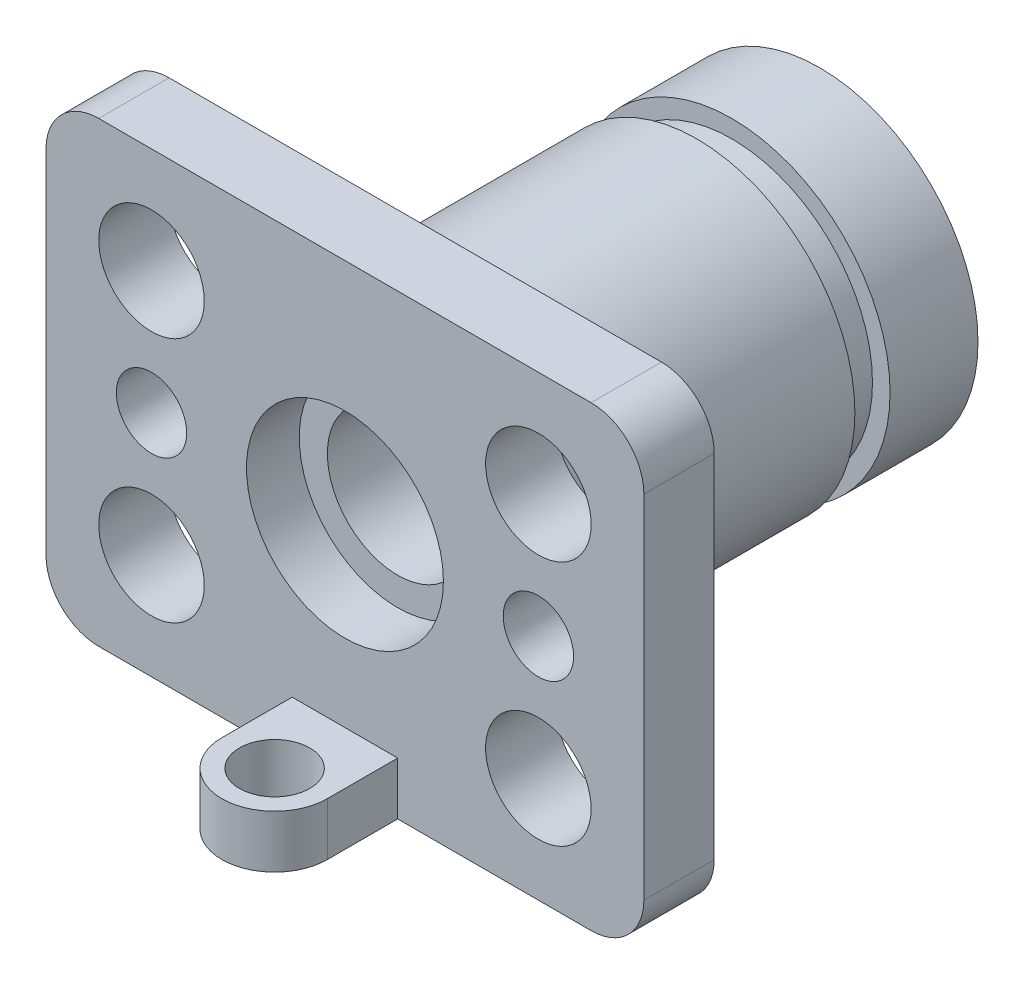
ISO-10303-21;
HEADER;
FILE_DESCRIPTION(('STEP AP214'),'2;1');
FILE_NAME('part.step','',(''),(''),'','','');
FILE_SCHEMA(('AUTOMOTIVE_DESIGN { 1 0 10303 214 1 1 1 1 }'));
ENDSEC;
DATA;
#1=APPLICATION_CONTEXT('core data for automotive mechanical design processes');
#2=APPLICATION_PROTOCOL_DEFINITION('international standard','automotive_design',2000,#1);
#3=PRODUCT_CONTEXT('',#1,'mechanical');
#4=PRODUCT('Part','Part','',(#3));
#5=PRODUCT_RELATED_PRODUCT_CATEGORY('part','',(#4));
#6=PRODUCT_DEFINITION_FORMATION('','',#4);
#7=PRODUCT_DEFINITION_CONTEXT('part definition',#1,'design');
#8=PRODUCT_DEFINITION('design','',#6,#7);
#9=PRODUCT_DEFINITION_SHAPE('','',#8);
#10=(LENGTH_UNIT() NAMED_UNIT(*) SI_UNIT(.MILLI.,.METRE.));
#11=(NAMED_UNIT(*) PLANE_ANGLE_UNIT() SI_UNIT($,.RADIAN.));
#12=(NAMED_UNIT(*) SI_UNIT($,.STERADIAN.) SOLID_ANGLE_UNIT());
#13=UNCERTAINTY_MEASURE_WITH_UNIT(LENGTH_MEASURE(1.E-05),#10,'distance_accuracy_value','');
#14=(GEOMETRIC_REPRESENTATION_CONTEXT(3) GLOBAL_UNCERTAINTY_ASSIGNED_CONTEXT((#13)) GLOBAL_UNIT_ASSIGNED_CONTEXT((#10,
#11,#12)) REPRESENTATION_CONTEXT('',''));
#15=CARTESIAN_POINT('',(0.,0.,0.));
#16=DIRECTION('',(0.,0.,1.));
#17=DIRECTION('',(1.,0.,0.));
#18=AXIS2_PLACEMENT_3D('',#15,#16,#17);
#19=CARTESIAN_POINT('',(0.,0.,25.));
#20=DIRECTION('',(0.,0.,-1.));
#21=DIRECTION('',(-1.,0.,0.));
#22=AXIS2_PLACEMENT_3D('',#19,#20,#21);
#23=CYLINDRICAL_SURFACE('',#22,45.);
#24=CARTESIAN_POINT('',(0.,0.,25.));
#25=DIRECTION('',(0.,0.,1.));
#26=DIRECTION('',(1.,0.,0.));
#27=AXIS2_PLACEMENT_3D('',#24,#25,#26);
#28=CIRCLE('',#27,45.);
#29=CARTESIAN_POINT('',(45.,0.,25.));
#30=VERTEX_POINT('',#29);
#31=EDGE_CURVE('E54',#30,#30,#28,.T.);
#32=ORIENTED_EDGE('',*,*,#31,.F.);
#33=EDGE_LOOP('',(#32));
#34=FACE_BOUND('',#33,.T.);
#35=CARTESIAN_POINT('',(0.,0.,0.));
#36=DIRECTION('',(0.,0.,1.));
#37=DIRECTION('',(1.,0.,0.));
#38=AXIS2_PLACEMENT_3D('',#35,#36,#37);
#39=CIRCLE('',#38,45.);
#40=CARTESIAN_POINT('',(45.,0.,0.));
#41=VERTEX_POINT('',#40);
#42=EDGE_CURVE('E284',#41,#41,#39,.T.);
#43=ORIENTED_EDGE('',*,*,#42,.T.);
#44=EDGE_LOOP('',(#43));
#45=FACE_BOUND('',#44,.T.);
#46=ADVANCED_FACE('F50',(#34,#45),#23,.T.);
#47=CARTESIAN_POINT('',(0.,0.,25.));
#48=DIRECTION('',(0.,0.,1.));
#49=DIRECTION('',(1.,0.,0.));
#50=AXIS2_PLACEMENT_3D('',#47,#48,#49);
#51=PLANE('',#50);
#52=CARTESIAN_POINT('',(0.,0.,25.));
#53=DIRECTION('',(0.,0.,1.));
#54=DIRECTION('',(1.,0.,0.));
#55=AXIS2_PLACEMENT_3D('',#52,#53,#54);
#56=CIRCLE('',#55,40.);
#57=CARTESIAN_POINT('',(40.,0.,25.));
#58=VERTEX_POINT('',#57);
#59=EDGE_CURVE('E11',#58,#58,#56,.T.);
#60=ORIENTED_EDGE('',*,*,#59,.F.);
#61=EDGE_LOOP('',(#60));
#62=FACE_BOUND('',#61,.T.);
#63=ORIENTED_EDGE('',*,*,#31,.T.);
#64=EDGE_LOOP('',(#63));
#65=FACE_BOUND('',#64,.T.);
#66=ADVANCED_FACE('F326',(#62,#65),#51,.T.);
#67=CARTESIAN_POINT('',(0.,0.,0.));
#68=DIRECTION('',(0.,0.,1.));
#69=DIRECTION('',(1.,0.,0.));
#70=AXIS2_PLACEMENT_3D('',#67,#68,#69);
#71=PLANE('',#70);
#72=CARTESIAN_POINT('',(0.,0.,0.));
#73=DIRECTION('',(0.,0.,1.));
#74=DIRECTION('',(1.,0.,0.));
#75=AXIS2_PLACEMENT_3D('',#72,#73,#74);
#76=CIRCLE('',#75,20.);
#77=CARTESIAN_POINT('',(20.,0.,0.));
#78=VERTEX_POINT('',#77);
#79=EDGE_CURVE('E202',#78,#78,#76,.T.);
#80=ORIENTED_EDGE('',*,*,#79,.T.);
#81=EDGE_LOOP('',(#80));
#82=FACE_BOUND('',#81,.T.);
#83=ORIENTED_EDGE('',*,*,#42,.F.);
#84=EDGE_LOOP('',(#83));
#85=FACE_BOUND('',#84,.T.);
#86=ADVANCED_FACE('F335',(#82,#85),#71,.F.);
#87=CARTESIAN_POINT('',(0.,0.,35.));
#88=DIRECTION('',(0.,0.,-1.));
#89=DIRECTION('',(-1.,0.,0.));
#90=AXIS2_PLACEMENT_3D('',#87,#88,#89);
#91=CYLINDRICAL_SURFACE('',#90,40.);
#92=CARTESIAN_POINT('',(0.,0.,35.));
#93=DIRECTION('',(0.,0.,1.));
#94=DIRECTION('',(1.,0.,0.));
#95=AXIS2_PLACEMENT_3D('',#92,#93,#94);
#96=CIRCLE('',#95,40.);
#97=CARTESIAN_POINT('',(40.,0.,35.));
#98=VERTEX_POINT('',#97);
#99=EDGE_CURVE('E279',#98,#98,#96,.T.);
#100=ORIENTED_EDGE('',*,*,#99,.F.);
#101=EDGE_LOOP('',(#100));
#102=FACE_BOUND('',#101,.T.);
#103=ORIENTED_EDGE('',*,*,#59,.T.);
#104=EDGE_LOOP('',(#103));
#105=FACE_BOUND('',#104,.T.);
#106=ADVANCED_FACE('F340',(#102,#105),#91,.T.);
#107=CARTESIAN_POINT('',(0.,0.,115.));
#108=DIRECTION('',(0.,0.,-1.));
#109=DIRECTION('',(-1.,0.,0.));
#110=AXIS2_PLACEMENT_3D('',#107,#108,#109);
#111=CYLINDRICAL_SURFACE('',#110,45.);
#112=CARTESIAN_POINT('',(0.,0.,115.));
#113=DIRECTION('',(0.,0.,1.));
#114=DIRECTION('',(1.,0.,0.));
#115=AXIS2_PLACEMENT_3D('',#112,#113,#114);
#116=CIRCLE('',#115,45.);
#117=CARTESIAN_POINT('',(45.,0.,115.));
#118=VERTEX_POINT('',#117);
#119=CARTESIAN_POINT('',(-45.,0.,115.));
#120=VERTEX_POINT('',#119);
#121=EDGE_CURVE('E274',#118,#120,#116,.T.);
#122=ORIENTED_EDGE('',*,*,#121,.F.);
#123=EDGE_CURVE('E276',#120,#118,#116,.T.);
#124=ORIENTED_EDGE('',*,*,#123,.F.);
#125=EDGE_LOOP('',(#122,#124));
#126=FACE_BOUND('',#125,.T.);
#127=CARTESIAN_POINT('',(0.,0.,35.));
#128=DIRECTION('',(0.,0.,1.));
#129=DIRECTION('',(1.,0.,0.));
#130=AXIS2_PLACEMENT_3D('',#127,#128,#129);
#131=CIRCLE('',#130,45.);
#132=CARTESIAN_POINT('',(45.,0.,35.));
#133=VERTEX_POINT('',#132);
#134=EDGE_CURVE('E273',#133,#133,#131,.T.);
#135=ORIENTED_EDGE('',*,*,#134,.T.);
#136=EDGE_LOOP('',(#135));
#137=FACE_BOUND('',#136,.T.);
#138=ADVANCED_FACE('F347',(#126,#137),#111,.T.);
#139=CARTESIAN_POINT('',(0.,0.,35.));
#140=DIRECTION('',(0.,0.,1.));
#141=DIRECTION('',(1.,0.,0.));
#142=AXIS2_PLACEMENT_3D('',#139,#140,#141);
#143=PLANE('',#142);
#144=ORIENTED_EDGE('',*,*,#99,.T.);
#145=EDGE_LOOP('',(#144));
#146=FACE_BOUND('',#145,.T.);
#147=ORIENTED_EDGE('',*,*,#134,.F.);
#148=EDGE_LOOP('',(#147));
#149=FACE_BOUND('',#148,.T.);
#150=ADVANCED_FACE('F351',(#146,#149),#143,.F.);
#151=CARTESIAN_POINT('',(70.,50.,135.));
#152=DIRECTION('',(0.,0.,-1.));
#153=DIRECTION('',(-1.,0.,0.));
#154=AXIS2_PLACEMENT_3D('',#151,#152,#153);
#155=CYLINDRICAL_SURFACE('',#154,15.);
#156=CARTESIAN_POINT('',(70.,50.,115.));
#157=DIRECTION('',(0.,0.,1.));
#158=DIRECTION('',(1.,0.,0.));
#159=AXIS2_PLACEMENT_3D('',#156,#157,#158);
#160=CIRCLE('',#159,15.);
#161=CARTESIAN_POINT('',(85.,49.9999999999999,115.));
#162=VERTEX_POINT('',#161);
#163=CARTESIAN_POINT('',(69.9999999999999,65.,115.));
#164=VERTEX_POINT('',#163);
#165=EDGE_CURVE('E207',#162,#164,#160,.T.);
#166=ORIENTED_EDGE('',*,*,#165,.T.);
#167=DIRECTION('',(0.,0.,-1.));
#168=VECTOR('',#167,1.);
#169=CARTESIAN_POINT('',(69.9999999999999,65.,135.));
#170=LINE('',#169,#168);
#171=CARTESIAN_POINT('',(69.9999999999999,65.,135.));
#172=VERTEX_POINT('',#171);
#173=EDGE_CURVE('E275',#172,#164,#170,.T.);
#174=ORIENTED_EDGE('',*,*,#173,.F.);
#175=CARTESIAN_POINT('',(70.,50.,135.));
#176=DIRECTION('',(0.,0.,1.));
#177=DIRECTION('',(1.,0.,0.));
#178=AXIS2_PLACEMENT_3D('',#175,#176,#177);
#179=CIRCLE('',#178,15.);
#180=CARTESIAN_POINT('',(85.,49.9999999999999,135.));
#181=VERTEX_POINT('',#180);
#182=EDGE_CURVE('E213',#181,#172,#179,.T.);
#183=ORIENTED_EDGE('',*,*,#182,.F.);
#184=DIRECTION('',(0.,0.,-1.));
#185=VECTOR('',#184,1.);
#186=CARTESIAN_POINT('',(85.,49.9999999999999,135.));
#187=LINE('',#186,#185);
#188=EDGE_CURVE('E237',#181,#162,#187,.T.);
#189=ORIENTED_EDGE('',*,*,#188,.T.);
#190=EDGE_LOOP('',(#166,#174,#183,#189));
#191=FACE_BOUND('',#190,.T.);
#192=ADVANCED_FACE('F355',(#191),#155,.T.);
#193=CARTESIAN_POINT('',(0.,65.,135.));
#194=DIRECTION('',(0.,1.,0.));
#195=DIRECTION('',(0.,0.,1.));
#196=AXIS2_PLACEMENT_3D('',#193,#194,#195);
#197=PLANE('',#196);
#198=DIRECTION('',(1.,0.,0.));
#199=VECTOR('',#198,1.);
#200=CARTESIAN_POINT('',(0.,65.,115.));
#201=LINE('',#200,#199);
#202=CARTESIAN_POINT('',(-69.9999999999999,65.,115.));
#203=VERTEX_POINT('',#202);
#204=EDGE_CURVE('E239',#203,#164,#201,.T.);
#205=ORIENTED_EDGE('',*,*,#204,.F.);
#206=DIRECTION('',(0.,0.,-1.));
#207=VECTOR('',#206,1.);
#208=CARTESIAN_POINT('',(-69.9999999999999,65.,135.));
#209=LINE('',#208,#207);
#210=CARTESIAN_POINT('',(-69.9999999999999,65.,135.));
#211=VERTEX_POINT('',#210);
#212=EDGE_CURVE('E269',#211,#203,#209,.T.);
#213=ORIENTED_EDGE('',*,*,#212,.F.);
#214=DIRECTION('',(1.,0.,0.));
#215=VECTOR('',#214,1.);
#216=CARTESIAN_POINT('',(0.,65.,135.));
#217=LINE('',#216,#215);
#218=EDGE_CURVE('E214',#211,#172,#217,.T.);
#219=ORIENTED_EDGE('',*,*,#218,.T.);
#220=ORIENTED_EDGE('',*,*,#173,.T.);
#221=EDGE_LOOP('',(#205,#213,#219,#220));
#222=FACE_BOUND('',#221,.T.);
#223=ADVANCED_FACE('F359',(#222),#197,.T.);
#224=CARTESIAN_POINT('',(-70.,50.,135.));
#225=DIRECTION('',(0.,0.,-1.));
#226=DIRECTION('',(-1.,0.,0.));
#227=AXIS2_PLACEMENT_3D('',#224,#225,#226);
#228=CYLINDRICAL_SURFACE('',#227,15.);
#229=CARTESIAN_POINT('',(-70.,50.,115.));
#230=DIRECTION('',(0.,0.,1.));
#231=DIRECTION('',(1.,0.,0.));
#232=AXIS2_PLACEMENT_3D('',#229,#230,#231);
#233=CIRCLE('',#232,15.);
#234=CARTESIAN_POINT('',(-85.,49.9999999999999,115.));
#235=VERTEX_POINT('',#234);
#236=EDGE_CURVE('E242',#203,#235,#233,.T.);
#237=ORIENTED_EDGE('',*,*,#236,.T.);
#238=DIRECTION('',(0.,0.,-1.));
#239=VECTOR('',#238,1.);
#240=CARTESIAN_POINT('',(-85.,49.9999999999999,135.));
#241=LINE('',#240,#239);
#242=CARTESIAN_POINT('',(-85.,49.9999999999999,135.));
#243=VERTEX_POINT('',#242);
#244=EDGE_CURVE('E268',#243,#235,#241,.T.);
#245=ORIENTED_EDGE('',*,*,#244,.F.);
#246=CARTESIAN_POINT('',(-70.,50.,135.));
#247=DIRECTION('',(0.,0.,1.));
#248=DIRECTION('',(1.,0.,0.));
#249=AXIS2_PLACEMENT_3D('',#246,#247,#248);
#250=CIRCLE('',#249,15.);
#251=EDGE_CURVE('E218',#211,#243,#250,.T.);
#252=ORIENTED_EDGE('',*,*,#251,.F.);
#253=ORIENTED_EDGE('',*,*,#212,.T.);
#254=EDGE_LOOP('',(#237,#245,#252,#253));
#255=FACE_BOUND('',#254,.T.);
#256=ADVANCED_FACE('F361',(#255),#228,.T.);
#257=CARTESIAN_POINT('',(-85.,0.,135.));
#258=DIRECTION('',(-1.,0.,0.));
#259=DIRECTION('',(0.,0.,1.));
#260=AXIS2_PLACEMENT_3D('',#257,#258,#259);
#261=PLANE('',#260);
#262=DIRECTION('',(0.,1.,0.));
#263=VECTOR('',#262,1.);
#264=CARTESIAN_POINT('',(-85.,0.,115.));
#265=LINE('',#264,#263);
#266=CARTESIAN_POINT('',(-85.,-49.9999999999999,115.));
#267=VERTEX_POINT('',#266);
#268=EDGE_CURVE('E245',#267,#235,#265,.T.);
#269=ORIENTED_EDGE('',*,*,#268,.F.);
#270=DIRECTION('',(0.,0.,-1.));
#271=VECTOR('',#270,1.);
#272=CARTESIAN_POINT('',(-85.,-49.9999999999999,135.));
#273=LINE('',#272,#271);
#274=CARTESIAN_POINT('',(-85.,-49.9999999999999,135.));
#275=VERTEX_POINT('',#274);
#276=EDGE_CURVE('E266',#275,#267,#273,.T.);
#277=ORIENTED_EDGE('',*,*,#276,.F.);
#278=DIRECTION('',(0.,1.,0.));
#279=VECTOR('',#278,1.);
#280=CARTESIAN_POINT('',(-85.,0.,135.));
#281=LINE('',#280,#279);
#282=EDGE_CURVE('E222',#275,#243,#281,.T.);
#283=ORIENTED_EDGE('',*,*,#282,.T.);
#284=ORIENTED_EDGE('',*,*,#244,.T.);
#285=EDGE_LOOP('',(#269,#277,#283,#284));
#286=FACE_BOUND('',#285,.T.);
#287=ADVANCED_FACE('F370',(#286),#261,.T.);
#288=CARTESIAN_POINT('',(-70.,-50.,135.));
#289=DIRECTION('',(0.,0.,-1.));
#290=DIRECTION('',(-1.,0.,0.));
#291=AXIS2_PLACEMENT_3D('',#288,#289,#290);
#292=CYLINDRICAL_SURFACE('',#291,15.);
#293=CARTESIAN_POINT('',(-70.,-50.,115.));
#294=DIRECTION('',(0.,0.,1.));
#295=DIRECTION('',(1.,0.,0.));
#296=AXIS2_PLACEMENT_3D('',#293,#294,#295);
#297=CIRCLE('',#296,15.);
#298=CARTESIAN_POINT('',(-69.9999999999999,-65.,115.));
#299=VERTEX_POINT('',#298);
#300=EDGE_CURVE('E246',#299,#267,#297,.F.);
#301=ORIENTED_EDGE('',*,*,#300,.F.);
#302=DIRECTION('',(0.,0.,-1.));
#303=VECTOR('',#302,1.);
#304=CARTESIAN_POINT('',(-69.9999999999999,-65.,135.));
#305=LINE('',#304,#303);
#306=CARTESIAN_POINT('',(-69.9999999999999,-65.,135.));
#307=VERTEX_POINT('',#306);
#308=EDGE_CURVE('E262',#307,#299,#305,.T.);
#309=ORIENTED_EDGE('',*,*,#308,.F.);
#310=CARTESIAN_POINT('',(-70.,-50.,135.));
#311=DIRECTION('',(0.,0.,1.));
#312=DIRECTION('',(1.,0.,0.));
#313=AXIS2_PLACEMENT_3D('',#310,#311,#312);
#314=CIRCLE('',#313,15.);
#315=EDGE_CURVE('E221',#307,#275,#314,.F.);
#316=ORIENTED_EDGE('',*,*,#315,.T.);
#317=ORIENTED_EDGE('',*,*,#276,.T.);
#318=EDGE_LOOP('',(#301,#309,#316,#317));
#319=FACE_BOUND('',#318,.T.);
#320=ADVANCED_FACE('F371',(#319),#292,.T.);
#321=CARTESIAN_POINT('',(0.,-65.,135.));
#322=DIRECTION('',(0.,-1.,0.));
#323=DIRECTION('',(0.,0.,-1.));
#324=AXIS2_PLACEMENT_3D('',#321,#322,#323);
#325=PLANE('',#324);
#326=CARTESIAN_POINT('',(0.,-65.,155.));
#327=DIRECTION('',(0.,1.,0.));
#328=DIRECTION('',(0.,0.,1.));
#329=AXIS2_PLACEMENT_3D('',#326,#327,#328);
#330=CIRCLE('',#329,10.);
#331=CARTESIAN_POINT('',(0.,-65.,165.));
#332=VERTEX_POINT('',#331);
#333=EDGE_CURVE('E180',#332,#332,#330,.T.);
#334=ORIENTED_EDGE('',*,*,#333,.T.);
#335=EDGE_LOOP('',(#334));
#336=FACE_BOUND('',#335,.T.);
#337=DIRECTION('',(-1.,0.,0.));
#338=VECTOR('',#337,1.);
#339=CARTESIAN_POINT('',(0.,-65.,115.));
#340=LINE('',#339,#338);
#341=CARTESIAN_POINT('',(69.9999999999999,-65.,115.));
#342=VERTEX_POINT('',#341);
#343=EDGE_CURVE('E253',#342,#299,#340,.T.);
#344=ORIENTED_EDGE('',*,*,#343,.F.);
#345=DIRECTION('',(0.,0.,-1.));
#346=VECTOR('',#345,1.);
#347=CARTESIAN_POINT('',(69.9999999999999,-65.,135.));
#348=LINE('',#347,#346);
#349=CARTESIAN_POINT('',(69.9999999999999,-65.,135.));
#350=VERTEX_POINT('',#349);
#351=EDGE_CURVE('E265',#350,#342,#348,.T.);
#352=ORIENTED_EDGE('',*,*,#351,.F.);
#353=DIRECTION('',(-1.,0.,0.));
#354=VECTOR('',#353,1.);
#355=CARTESIAN_POINT('',(0.,-65.,135.));
#356=LINE('',#355,#354);
#357=CARTESIAN_POINT('',(15.,-65.,135.));
#358=VERTEX_POINT('',#357);
#359=EDGE_CURVE('E229',#350,#358,#356,.T.);
#360=ORIENTED_EDGE('',*,*,#359,.T.);
#361=DIRECTION('',(0.,0.,1.));
#362=VECTOR('',#361,1.);
#363=CARTESIAN_POINT('',(15.,-65.,155.));
#364=LINE('',#363,#362);
#365=CARTESIAN_POINT('',(15.,-65.,155.));
#366=VERTEX_POINT('',#365);
#367=EDGE_CURVE('E64',#358,#366,#364,.T.);
#368=ORIENTED_EDGE('',*,*,#367,.T.);
#369=CARTESIAN_POINT('',(0.,-65.,155.));
#370=DIRECTION('',(0.,-1.,0.));
#371=DIRECTION('',(0.,0.,-1.));
#372=AXIS2_PLACEMENT_3D('',#369,#370,#371);
#373=CIRCLE('',#372,15.);
#374=CARTESIAN_POINT('',(-15.,-65.,155.));
#375=VERTEX_POINT('',#374);
#376=EDGE_CURVE('E175',#366,#375,#373,.T.);
#377=ORIENTED_EDGE('',*,*,#376,.T.);
#378=DIRECTION('',(0.,0.,-1.));
#379=VECTOR('',#378,1.);
#380=CARTESIAN_POINT('',(-15.,-65.,155.));
#381=LINE('',#380,#379);
#382=CARTESIAN_POINT('',(-15.,-65.,135.));
#383=VERTEX_POINT('',#382);
#384=EDGE_CURVE('E146',#375,#383,#381,.T.);
#385=ORIENTED_EDGE('',*,*,#384,.T.);
#386=EDGE_CURVE('E227',#383,#307,#356,.T.);
#387=ORIENTED_EDGE('',*,*,#386,.T.);
#388=ORIENTED_EDGE('',*,*,#308,.T.);
#389=EDGE_LOOP('',(#344,#352,#360,#368,#377,#385,#387,#388));
#390=FACE_BOUND('',#389,.T.);
#391=ADVANCED_FACE('F374',(#336,#390),#325,.T.);
#392=CARTESIAN_POINT('',(70.,-50.,135.));
#393=DIRECTION('',(0.,0.,-1.));
#394=DIRECTION('',(-1.,0.,0.));
#395=AXIS2_PLACEMENT_3D('',#392,#393,#394);
#396=CYLINDRICAL_SURFACE('',#395,15.);
#397=CARTESIAN_POINT('',(70.,-50.,115.));
#398=DIRECTION('',(0.,0.,1.));
#399=DIRECTION('',(1.,0.,0.));
#400=AXIS2_PLACEMENT_3D('',#397,#398,#399);
#401=CIRCLE('',#400,15.);
#402=CARTESIAN_POINT('',(85.,-49.9999999999999,115.));
#403=VERTEX_POINT('',#402);
#404=EDGE_CURVE('E255',#342,#403,#401,.T.);
#405=ORIENTED_EDGE('',*,*,#404,.T.);
#406=DIRECTION('',(0.,0.,-1.));
#407=VECTOR('',#406,1.);
#408=CARTESIAN_POINT('',(85.,-49.9999999999999,135.));
#409=LINE('',#408,#407);
#410=CARTESIAN_POINT('',(85.,-49.9999999999999,135.));
#411=VERTEX_POINT('',#410);
#412=EDGE_CURVE('E257',#411,#403,#409,.T.);
#413=ORIENTED_EDGE('',*,*,#412,.F.);
#414=CARTESIAN_POINT('',(70.,-50.,135.));
#415=DIRECTION('',(0.,0.,1.));
#416=DIRECTION('',(1.,0.,0.));
#417=AXIS2_PLACEMENT_3D('',#414,#415,#416);
#418=CIRCLE('',#417,15.);
#419=EDGE_CURVE('E233',#350,#411,#418,.T.);
#420=ORIENTED_EDGE('',*,*,#419,.F.);
#421=ORIENTED_EDGE('',*,*,#351,.T.);
#422=EDGE_LOOP('',(#405,#413,#420,#421));
#423=FACE_BOUND('',#422,.T.);
#424=ADVANCED_FACE('F377',(#423),#396,.T.);
#425=CARTESIAN_POINT('',(85.,0.,135.));
#426=DIRECTION('',(1.,0.,0.));
#427=DIRECTION('',(0.,0.,-1.));
#428=AXIS2_PLACEMENT_3D('',#425,#426,#427);
#429=PLANE('',#428);
#430=DIRECTION('',(0.,-1.,0.));
#431=VECTOR('',#430,1.);
#432=CARTESIAN_POINT('',(85.,0.,115.));
#433=LINE('',#432,#431);
#434=EDGE_CURVE('E216',#162,#403,#433,.T.);
#435=ORIENTED_EDGE('',*,*,#434,.F.);
#436=ORIENTED_EDGE('',*,*,#188,.F.);
#437=DIRECTION('',(0.,-1.,0.));
#438=VECTOR('',#437,1.);
#439=CARTESIAN_POINT('',(85.,0.,135.));
#440=LINE('',#439,#438);
#441=EDGE_CURVE('E231',#181,#411,#440,.T.);
#442=ORIENTED_EDGE('',*,*,#441,.T.);
#443=ORIENTED_EDGE('',*,*,#412,.T.);
#444=EDGE_LOOP('',(#435,#436,#442,#443));
#445=FACE_BOUND('',#444,.T.);
#446=ADVANCED_FACE('F382',(#445),#429,.T.);
#447=CARTESIAN_POINT('',(0.,0.,135.));
#448=DIRECTION('',(0.,0.,1.));
#449=DIRECTION('',(1.,0.,0.));
#450=AXIS2_PLACEMENT_3D('',#447,#448,#449);
#451=PLANE('',#450);
#452=DIRECTION('',(0.,-1.,0.));
#453=VECTOR('',#452,1.);
#454=CARTESIAN_POINT('',(-15.,-50.,135.));
#455=LINE('',#454,#453);
#456=CARTESIAN_POINT('',(-15.,-50.,135.));
#457=VERTEX_POINT('',#456);
#458=EDGE_CURVE('E153',#457,#383,#455,.T.);
#459=ORIENTED_EDGE('',*,*,#458,.F.);
#460=DIRECTION('',(1.,0.,0.));
#461=VECTOR('',#460,1.);
#462=CARTESIAN_POINT('',(-15.,-50.,135.));
#463=LINE('',#462,#461);
#464=CARTESIAN_POINT('',(15.,-50.,135.));
#465=VERTEX_POINT('',#464);
#466=EDGE_CURVE('E162',#457,#465,#463,.T.);
#467=ORIENTED_EDGE('',*,*,#466,.T.);
#468=DIRECTION('',(0.,-1.,0.));
#469=VECTOR('',#468,1.);
#470=CARTESIAN_POINT('',(15.,-50.,135.));
#471=LINE('',#470,#469);
#472=EDGE_CURVE('E182',#465,#358,#471,.T.);
#473=ORIENTED_EDGE('',*,*,#472,.T.);
#474=ORIENTED_EDGE('',*,*,#359,.F.);
#475=ORIENTED_EDGE('',*,*,#419,.T.);
#476=ORIENTED_EDGE('',*,*,#441,.F.);
#477=ORIENTED_EDGE('',*,*,#182,.T.);
#478=ORIENTED_EDGE('',*,*,#218,.F.);
#479=ORIENTED_EDGE('',*,*,#251,.T.);
#480=ORIENTED_EDGE('',*,*,#282,.F.);
#481=ORIENTED_EDGE('',*,*,#315,.F.);
#482=ORIENTED_EDGE('',*,*,#386,.F.);
#483=EDGE_LOOP('',(#459,#467,#473,#474,#475,#476,#477,#478,#479,#480,#481,#482));
#484=FACE_BOUND('',#483,.T.);
#485=CARTESIAN_POINT('',(55.,35.,135.));
#486=DIRECTION('',(0.,0.,1.));
#487=DIRECTION('',(1.,0.,0.));
#488=AXIS2_PLACEMENT_3D('',#485,#486,#487);
#489=CIRCLE('',#488,15.);
#490=CARTESIAN_POINT('',(70.,35.,135.));
#491=VERTEX_POINT('',#490);
#492=EDGE_CURVE('E177',#491,#491,#489,.T.);
#493=ORIENTED_EDGE('',*,*,#492,.F.);
#494=EDGE_LOOP('',(#493));
#495=FACE_BOUND('',#494,.T.);
#496=CARTESIAN_POINT('',(55.,0.,135.));
#497=DIRECTION('',(0.,0.,1.));
#498=DIRECTION('',(1.,0.,0.));
#499=AXIS2_PLACEMENT_3D('',#496,#497,#498);
#500=CIRCLE('',#499,10.);
#501=CARTESIAN_POINT('',(65.,0.,135.));
#502=VERTEX_POINT('',#501);
#503=EDGE_CURVE('E194',#502,#502,#500,.T.);
#504=ORIENTED_EDGE('',*,*,#503,.F.);
#505=EDGE_LOOP('',(#504));
#506=FACE_BOUND('',#505,.T.);
#507=CARTESIAN_POINT('',(55.,-35.,135.));
#508=DIRECTION('',(0.,0.,1.));
#509=DIRECTION('',(1.,0.,0.));
#510=AXIS2_PLACEMENT_3D('',#507,#508,#509);
#511=CIRCLE('',#510,15.);
#512=CARTESIAN_POINT('',(70.,-35.,135.));
#513=VERTEX_POINT('',#512);
#514=EDGE_CURVE('E193',#513,#513,#511,.T.);
#515=ORIENTED_EDGE('',*,*,#514,.F.);
#516=EDGE_LOOP('',(#515));
#517=FACE_BOUND('',#516,.T.);
#518=CARTESIAN_POINT('',(-55.,-35.,135.));
#519=DIRECTION('',(0.,0.,1.));
#520=DIRECTION('',(1.,0.,0.));
#521=AXIS2_PLACEMENT_3D('',#518,#519,#520);
#522=CIRCLE('',#521,15.);
#523=CARTESIAN_POINT('',(-40.,-35.,135.));
#524=VERTEX_POINT('',#523);
#525=EDGE_CURVE('E189',#524,#524,#522,.T.);
#526=ORIENTED_EDGE('',*,*,#525,.F.);
#527=EDGE_LOOP('',(#526));
#528=FACE_BOUND('',#527,.T.);
#529=CARTESIAN_POINT('',(-55.,0.,135.));
#530=DIRECTION('',(0.,0.,1.));
#531=DIRECTION('',(1.,0.,0.));
#532=AXIS2_PLACEMENT_3D('',#529,#530,#531);
#533=CIRCLE('',#532,10.);
#534=CARTESIAN_POINT('',(-45.,0.,135.));
#535=VERTEX_POINT('',#534);
#536=EDGE_CURVE('E184',#535,#535,#533,.T.);
#537=ORIENTED_EDGE('',*,*,#536,.F.);
#538=EDGE_LOOP('',(#537));
#539=FACE_BOUND('',#538,.T.);
#540=CARTESIAN_POINT('',(-55.,35.,135.));
#541=DIRECTION('',(0.,0.,1.));
#542=DIRECTION('',(1.,0.,0.));
#543=AXIS2_PLACEMENT_3D('',#540,#541,#542);
#544=CIRCLE('',#543,15.);
#545=CARTESIAN_POINT('',(-40.,35.,135.));
#546=VERTEX_POINT('',#545);
#547=EDGE_CURVE('E187',#546,#546,#544,.T.);
#548=ORIENTED_EDGE('',*,*,#547,.F.);
#549=EDGE_LOOP('',(#548));
#550=FACE_BOUND('',#549,.T.);
#551=CARTESIAN_POINT('',(0.,0.,135.));
#552=DIRECTION('',(0.,0.,1.));
#553=DIRECTION('',(1.,0.,0.));
#554=AXIS2_PLACEMENT_3D('',#551,#552,#553);
#555=CIRCLE('',#554,28.);
#556=CARTESIAN_POINT('',(28.,0.,135.));
#557=VERTEX_POINT('',#556);
#558=EDGE_CURVE('E209',#557,#557,#555,.T.);
#559=ORIENTED_EDGE('',*,*,#558,.F.);
#560=EDGE_LOOP('',(#559));
#561=FACE_BOUND('',#560,.T.);
#562=ADVANCED_FACE('F390',(#484,#495,#506,#517,#528,#539,#550,#561),#451,.T.);
#563=CARTESIAN_POINT('',(0.,0.,115.));
#564=DIRECTION('',(0.,0.,1.));
#565=DIRECTION('',(1.,0.,0.));
#566=AXIS2_PLACEMENT_3D('',#563,#564,#565);
#567=PLANE('',#566);
#568=CARTESIAN_POINT('',(55.,35.,115.));
#569=DIRECTION('',(0.,0.,1.));
#570=DIRECTION('',(1.,0.,0.));
#571=AXIS2_PLACEMENT_3D('',#568,#569,#570);
#572=CIRCLE('',#571,15.);
#573=CARTESIAN_POINT('',(70.,35.,115.));
#574=VERTEX_POINT('',#573);
#575=EDGE_CURVE('E49',#574,#574,#572,.T.);
#576=ORIENTED_EDGE('',*,*,#575,.T.);
#577=EDGE_LOOP('',(#576));
#578=FACE_BOUND('',#577,.T.);
#579=CARTESIAN_POINT('',(55.,-35.,115.));
#580=DIRECTION('',(0.,0.,1.));
#581=DIRECTION('',(1.,0.,0.));
#582=AXIS2_PLACEMENT_3D('',#579,#580,#581);
#583=CIRCLE('',#582,15.);
#584=CARTESIAN_POINT('',(70.,-35.,115.));
#585=VERTEX_POINT('',#584);
#586=EDGE_CURVE('E297',#585,#585,#583,.T.);
#587=ORIENTED_EDGE('',*,*,#586,.T.);
#588=EDGE_LOOP('',(#587));
#589=FACE_BOUND('',#588,.T.);
#590=CARTESIAN_POINT('',(-55.,-35.,115.));
#591=DIRECTION('',(0.,0.,1.));
#592=DIRECTION('',(1.,0.,0.));
#593=AXIS2_PLACEMENT_3D('',#590,#591,#592);
#594=CIRCLE('',#593,15.);
#595=CARTESIAN_POINT('',(-40.,-35.,115.));
#596=VERTEX_POINT('',#595);
#597=EDGE_CURVE('E294',#596,#596,#594,.T.);
#598=ORIENTED_EDGE('',*,*,#597,.T.);
#599=EDGE_LOOP('',(#598));
#600=FACE_BOUND('',#599,.T.);
#601=CARTESIAN_POINT('',(-55.,35.,115.));
#602=DIRECTION('',(0.,0.,1.));
#603=DIRECTION('',(1.,0.,0.));
#604=AXIS2_PLACEMENT_3D('',#601,#602,#603);
#605=CIRCLE('',#604,15.);
#606=CARTESIAN_POINT('',(-40.,35.,115.));
#607=VERTEX_POINT('',#606);
#608=EDGE_CURVE('E203',#607,#607,#605,.T.);
#609=ORIENTED_EDGE('',*,*,#608,.T.);
#610=EDGE_LOOP('',(#609));
#611=FACE_BOUND('',#610,.T.);
#612=ORIENTED_EDGE('',*,*,#123,.T.);
#613=CARTESIAN_POINT('',(55.,0.,115.));
#614=DIRECTION('',(0.,0.,1.));
#615=DIRECTION('',(1.,0.,0.));
#616=AXIS2_PLACEMENT_3D('',#613,#614,#615);
#617=CIRCLE('',#616,10.);
#618=EDGE_CURVE('E298',#118,#118,#617,.T.);
#619=ORIENTED_EDGE('',*,*,#618,.T.);
#620=ORIENTED_EDGE('',*,*,#121,.T.);
#621=CARTESIAN_POINT('',(-55.,0.,115.));
#622=DIRECTION('',(0.,0.,1.));
#623=DIRECTION('',(1.,0.,0.));
#624=AXIS2_PLACEMENT_3D('',#621,#622,#623);
#625=CIRCLE('',#624,10.);
#626=EDGE_CURVE('E69',#120,#120,#625,.T.);
#627=ORIENTED_EDGE('',*,*,#626,.T.);
#628=EDGE_LOOP('',(#612,#619,#620,#627));
#629=FACE_BOUND('',#628,.T.);
#630=ORIENTED_EDGE('',*,*,#165,.F.);
#631=ORIENTED_EDGE('',*,*,#434,.T.);
#632=ORIENTED_EDGE('',*,*,#404,.F.);
#633=ORIENTED_EDGE('',*,*,#343,.T.);
#634=ORIENTED_EDGE('',*,*,#300,.T.);
#635=ORIENTED_EDGE('',*,*,#268,.T.);
#636=ORIENTED_EDGE('',*,*,#236,.F.);
#637=ORIENTED_EDGE('',*,*,#204,.T.);
#638=EDGE_LOOP('',(#630,#631,#632,#633,#634,#635,#636,#637));
#639=FACE_BOUND('',#638,.T.);
#640=ADVANCED_FACE('F308',(#578,#589,#600,#611,#629,#639),#567,.F.);
#641=CARTESIAN_POINT('',(0.,0.,120.));
#642=DIRECTION('',(0.,0.,1.));
#643=DIRECTION('',(1.,0.,0.));
#644=AXIS2_PLACEMENT_3D('',#641,#642,#643);
#645=CYLINDRICAL_SURFACE('',#644,28.);
#646=CARTESIAN_POINT('',(0.,0.,120.));
#647=DIRECTION('',(0.,0.,1.));
#648=DIRECTION('',(1.,0.,0.));
#649=AXIS2_PLACEMENT_3D('',#646,#647,#648);
#650=CIRCLE('',#649,28.);
#651=CARTESIAN_POINT('',(28.,0.,120.));
#652=VERTEX_POINT('',#651);
#653=EDGE_CURVE('E206',#652,#652,#650,.T.);
#654=ORIENTED_EDGE('',*,*,#653,.F.);
#655=EDGE_LOOP('',(#654));
#656=FACE_BOUND('',#655,.T.);
#657=ORIENTED_EDGE('',*,*,#558,.T.);
#658=EDGE_LOOP('',(#657));
#659=FACE_BOUND('',#658,.T.);
#660=ADVANCED_FACE('F391',(#656,#659),#645,.F.);
#661=CARTESIAN_POINT('',(0.,0.,120.));
#662=DIRECTION('',(0.,0.,1.));
#663=DIRECTION('',(1.,0.,0.));
#664=AXIS2_PLACEMENT_3D('',#661,#662,#663);
#665=PLANE('',#664);
#666=CARTESIAN_POINT('',(0.,0.,120.));
#667=DIRECTION('',(0.,0.,1.));
#668=DIRECTION('',(1.,0.,0.));
#669=AXIS2_PLACEMENT_3D('',#666,#667,#668);
#670=CIRCLE('',#669,20.);
#671=CARTESIAN_POINT('',(20.,0.,120.));
#672=VERTEX_POINT('',#671);
#673=EDGE_CURVE('E205',#672,#672,#670,.T.);
#674=ORIENTED_EDGE('',*,*,#673,.F.);
#675=EDGE_LOOP('',(#674));
#676=FACE_BOUND('',#675,.T.);
#677=ORIENTED_EDGE('',*,*,#653,.T.);
#678=EDGE_LOOP('',(#677));
#679=FACE_BOUND('',#678,.T.);
#680=ADVANCED_FACE('F400',(#676,#679),#665,.T.);
#681=CARTESIAN_POINT('',(0.,0.,-30.));
#682=DIRECTION('',(0.,0.,1.));
#683=DIRECTION('',(1.,0.,0.));
#684=AXIS2_PLACEMENT_3D('',#681,#682,#683);
#685=CYLINDRICAL_SURFACE('',#684,20.);
#686=ORIENTED_EDGE('',*,*,#673,.T.);
#687=EDGE_LOOP('',(#686));
#688=FACE_BOUND('',#687,.T.);
#689=ORIENTED_EDGE('',*,*,#79,.F.);
#690=EDGE_LOOP('',(#689));
#691=FACE_BOUND('',#690,.T.);
#692=ADVANCED_FACE('F402',(#688,#691),#685,.F.);
#693=CARTESIAN_POINT('',(-55.,35.,-15.));
#694=DIRECTION('',(0.,0.,1.));
#695=DIRECTION('',(1.,0.,0.));
#696=AXIS2_PLACEMENT_3D('',#693,#694,#695);
#697=CYLINDRICAL_SURFACE('',#696,15.);
#698=ORIENTED_EDGE('',*,*,#547,.T.);
#699=EDGE_LOOP('',(#698));
#700=FACE_BOUND('',#699,.T.);
#701=ORIENTED_EDGE('',*,*,#608,.F.);
#702=EDGE_LOOP('',(#701));
#703=FACE_BOUND('',#702,.T.);
#704=ADVANCED_FACE('F404',(#700,#703),#697,.F.);
#705=CARTESIAN_POINT('',(-55.,0.,-15.));
#706=DIRECTION('',(0.,0.,1.));
#707=DIRECTION('',(1.,0.,0.));
#708=AXIS2_PLACEMENT_3D('',#705,#706,#707);
#709=CYLINDRICAL_SURFACE('',#708,10.);
#710=ORIENTED_EDGE('',*,*,#536,.T.);
#711=EDGE_LOOP('',(#710));
#712=FACE_BOUND('',#711,.T.);
#713=ORIENTED_EDGE('',*,*,#626,.F.);
#714=EDGE_LOOP('',(#713));
#715=FACE_BOUND('',#714,.T.);
#716=ADVANCED_FACE('F407',(#712,#715),#709,.F.);
#717=CARTESIAN_POINT('',(-55.,-35.,-15.));
#718=DIRECTION('',(0.,0.,1.));
#719=DIRECTION('',(1.,0.,0.));
#720=AXIS2_PLACEMENT_3D('',#717,#718,#719);
#721=CYLINDRICAL_SURFACE('',#720,15.);
#722=ORIENTED_EDGE('',*,*,#525,.T.);
#723=EDGE_LOOP('',(#722));
#724=FACE_BOUND('',#723,.T.);
#725=ORIENTED_EDGE('',*,*,#597,.F.);
#726=EDGE_LOOP('',(#725));
#727=FACE_BOUND('',#726,.T.);
#728=ADVANCED_FACE('F415',(#724,#727),#721,.F.);
#729=CARTESIAN_POINT('',(55.,-35.,-15.));
#730=DIRECTION('',(0.,0.,1.));
#731=DIRECTION('',(1.,0.,0.));
#732=AXIS2_PLACEMENT_3D('',#729,#730,#731);
#733=CYLINDRICAL_SURFACE('',#732,15.);
#734=ORIENTED_EDGE('',*,*,#514,.T.);
#735=EDGE_LOOP('',(#734));
#736=FACE_BOUND('',#735,.T.);
#737=ORIENTED_EDGE('',*,*,#586,.F.);
#738=EDGE_LOOP('',(#737));
#739=FACE_BOUND('',#738,.T.);
#740=ADVANCED_FACE('F321',(#736,#739),#733,.F.);
#741=CARTESIAN_POINT('',(55.,0.,-15.));
#742=DIRECTION('',(0.,0.,1.));
#743=DIRECTION('',(1.,0.,0.));
#744=AXIS2_PLACEMENT_3D('',#741,#742,#743);
#745=CYLINDRICAL_SURFACE('',#744,10.);
#746=ORIENTED_EDGE('',*,*,#503,.T.);
#747=EDGE_LOOP('',(#746));
#748=FACE_BOUND('',#747,.T.);
#749=ORIENTED_EDGE('',*,*,#618,.F.);
#750=EDGE_LOOP('',(#749));
#751=FACE_BOUND('',#750,.T.);
#752=ADVANCED_FACE('F313',(#748,#751),#745,.F.);
#753=CARTESIAN_POINT('',(55.,35.,-15.));
#754=DIRECTION('',(0.,0.,1.));
#755=DIRECTION('',(1.,0.,0.));
#756=AXIS2_PLACEMENT_3D('',#753,#754,#755);
#757=CYLINDRICAL_SURFACE('',#756,15.);
#758=ORIENTED_EDGE('',*,*,#492,.T.);
#759=EDGE_LOOP('',(#758));
#760=FACE_BOUND('',#759,.T.);
#761=ORIENTED_EDGE('',*,*,#575,.F.);
#762=EDGE_LOOP('',(#761));
#763=FACE_BOUND('',#762,.T.);
#764=ADVANCED_FACE('F310',(#760,#763),#757,.F.);
#765=CARTESIAN_POINT('',(0.,-50.,155.));
#766=DIRECTION('',(0.,-1.,0.));
#767=DIRECTION('',(0.,0.,-1.));
#768=AXIS2_PLACEMENT_3D('',#765,#766,#767);
#769=CYLINDRICAL_SURFACE('',#768,15.);
#770=ORIENTED_EDGE('',*,*,#376,.F.);
#771=DIRECTION('',(0.,-1.,0.));
#772=VECTOR('',#771,1.);
#773=CARTESIAN_POINT('',(15.,-50.,155.));
#774=LINE('',#773,#772);
#775=CARTESIAN_POINT('',(15.,-50.,155.));
#776=VERTEX_POINT('',#775);
#777=EDGE_CURVE('E167',#776,#366,#774,.T.);
#778=ORIENTED_EDGE('',*,*,#777,.F.);
#779=CARTESIAN_POINT('',(0.,-50.,155.));
#780=DIRECTION('',(0.,-1.,0.));
#781=DIRECTION('',(0.,0.,-1.));
#782=AXIS2_PLACEMENT_3D('',#779,#780,#781);
#783=CIRCLE('',#782,15.);
#784=CARTESIAN_POINT('',(-15.,-50.,155.));
#785=VERTEX_POINT('',#784);
#786=EDGE_CURVE('E159',#776,#785,#783,.T.);
#787=ORIENTED_EDGE('',*,*,#786,.T.);
#788=DIRECTION('',(0.,-1.,0.));
#789=VECTOR('',#788,1.);
#790=CARTESIAN_POINT('',(-15.,-50.,155.));
#791=LINE('',#790,#789);
#792=EDGE_CURVE('E142',#785,#375,#791,.T.);
#793=ORIENTED_EDGE('',*,*,#792,.T.);
#794=EDGE_LOOP('',(#770,#778,#787,#793));
#795=FACE_BOUND('',#794,.T.);
#796=ADVANCED_FACE('F164',(#795),#769,.T.);
#797=CARTESIAN_POINT('',(15.,-50.,155.));
#798=DIRECTION('',(1.,0.,0.));
#799=DIRECTION('',(0.,0.,-1.));
#800=AXIS2_PLACEMENT_3D('',#797,#798,#799);
#801=PLANE('',#800);
#802=ORIENTED_EDGE('',*,*,#367,.F.);
#803=ORIENTED_EDGE('',*,*,#472,.F.);
#804=DIRECTION('',(0.,0.,1.));
#805=VECTOR('',#804,1.);
#806=CARTESIAN_POINT('',(15.,-50.,155.));
#807=LINE('',#806,#805);
#808=EDGE_CURVE('E152',#465,#776,#807,.T.);
#809=ORIENTED_EDGE('',*,*,#808,.T.);
#810=ORIENTED_EDGE('',*,*,#777,.T.);
#811=EDGE_LOOP('',(#802,#803,#809,#810));
#812=FACE_BOUND('',#811,.T.);
#813=ADVANCED_FACE('F317',(#812),#801,.T.);
#814=CARTESIAN_POINT('',(-15.,-50.,155.));
#815=DIRECTION('',(-1.,0.,0.));
#816=DIRECTION('',(0.,0.,1.));
#817=AXIS2_PLACEMENT_3D('',#814,#815,#816);
#818=PLANE('',#817);
#819=ORIENTED_EDGE('',*,*,#384,.F.);
#820=ORIENTED_EDGE('',*,*,#792,.F.);
#821=DIRECTION('',(0.,0.,-1.));
#822=VECTOR('',#821,1.);
#823=CARTESIAN_POINT('',(-15.,-50.,155.));
#824=LINE('',#823,#822);
#825=EDGE_CURVE('E144',#785,#457,#824,.T.);
#826=ORIENTED_EDGE('',*,*,#825,.T.);
#827=ORIENTED_EDGE('',*,*,#458,.T.);
#828=EDGE_LOOP('',(#819,#820,#826,#827));
#829=FACE_BOUND('',#828,.T.);
#830=ADVANCED_FACE('F145',(#829),#818,.T.);
#831=CARTESIAN_POINT('',(0.,-50.,155.));
#832=DIRECTION('',(0.,-1.,0.));
#833=DIRECTION('',(0.,0.,-1.));
#834=AXIS2_PLACEMENT_3D('',#831,#832,#833);
#835=PLANE('',#834);
#836=CARTESIAN_POINT('',(0.,-50.,155.));
#837=DIRECTION('',(0.,1.,0.));
#838=DIRECTION('',(0.,0.,1.));
#839=AXIS2_PLACEMENT_3D('',#836,#837,#838);
#840=CIRCLE('',#839,10.);
#841=CARTESIAN_POINT('',(0.,-50.,165.));
#842=VERTEX_POINT('',#841);
#843=EDGE_CURVE('E168',#842,#842,#840,.T.);
#844=ORIENTED_EDGE('',*,*,#843,.F.);
#845=EDGE_LOOP('',(#844));
#846=FACE_BOUND('',#845,.T.);
#847=ORIENTED_EDGE('',*,*,#786,.F.);
#848=ORIENTED_EDGE('',*,*,#808,.F.);
#849=ORIENTED_EDGE('',*,*,#466,.F.);
#850=ORIENTED_EDGE('',*,*,#825,.F.);
#851=EDGE_LOOP('',(#847,#848,#849,#850));
#852=FACE_BOUND('',#851,.T.);
#853=ADVANCED_FACE('F158',(#846,#852),#835,.F.);
#854=CARTESIAN_POINT('',(0.,-65.,155.));
#855=DIRECTION('',(0.,1.,0.));
#856=DIRECTION('',(0.,0.,1.));
#857=AXIS2_PLACEMENT_3D('',#854,#855,#856);
#858=CYLINDRICAL_SURFACE('',#857,10.);
#859=ORIENTED_EDGE('',*,*,#333,.F.);
#860=EDGE_LOOP('',(#859));
#861=FACE_BOUND('',#860,.T.);
#862=ORIENTED_EDGE('',*,*,#843,.T.);
#863=EDGE_LOOP('',(#862));
#864=FACE_BOUND('',#863,.T.);
#865=ADVANCED_FACE('F495',(#861,#864),#858,.F.);
#866=CLOSED_SHELL('',(#46,#66,#86,#106,#138,#150,#192,#223,#256,#287,#320,#391,#424,#446,#562,
#640,#660,#680,#692,#704,#716,#728,#740,#752,#764,#796,#813,#830,#853,#865));
#867=MANIFOLD_SOLID_BREP('B2',#866);
#868=ADVANCED_BREP_SHAPE_REPRESENTATION('',(#18,#867),#14);
#869=SHAPE_DEFINITION_REPRESENTATION(#9,#868);
ENDSEC;
END-ISO-10303-21;
